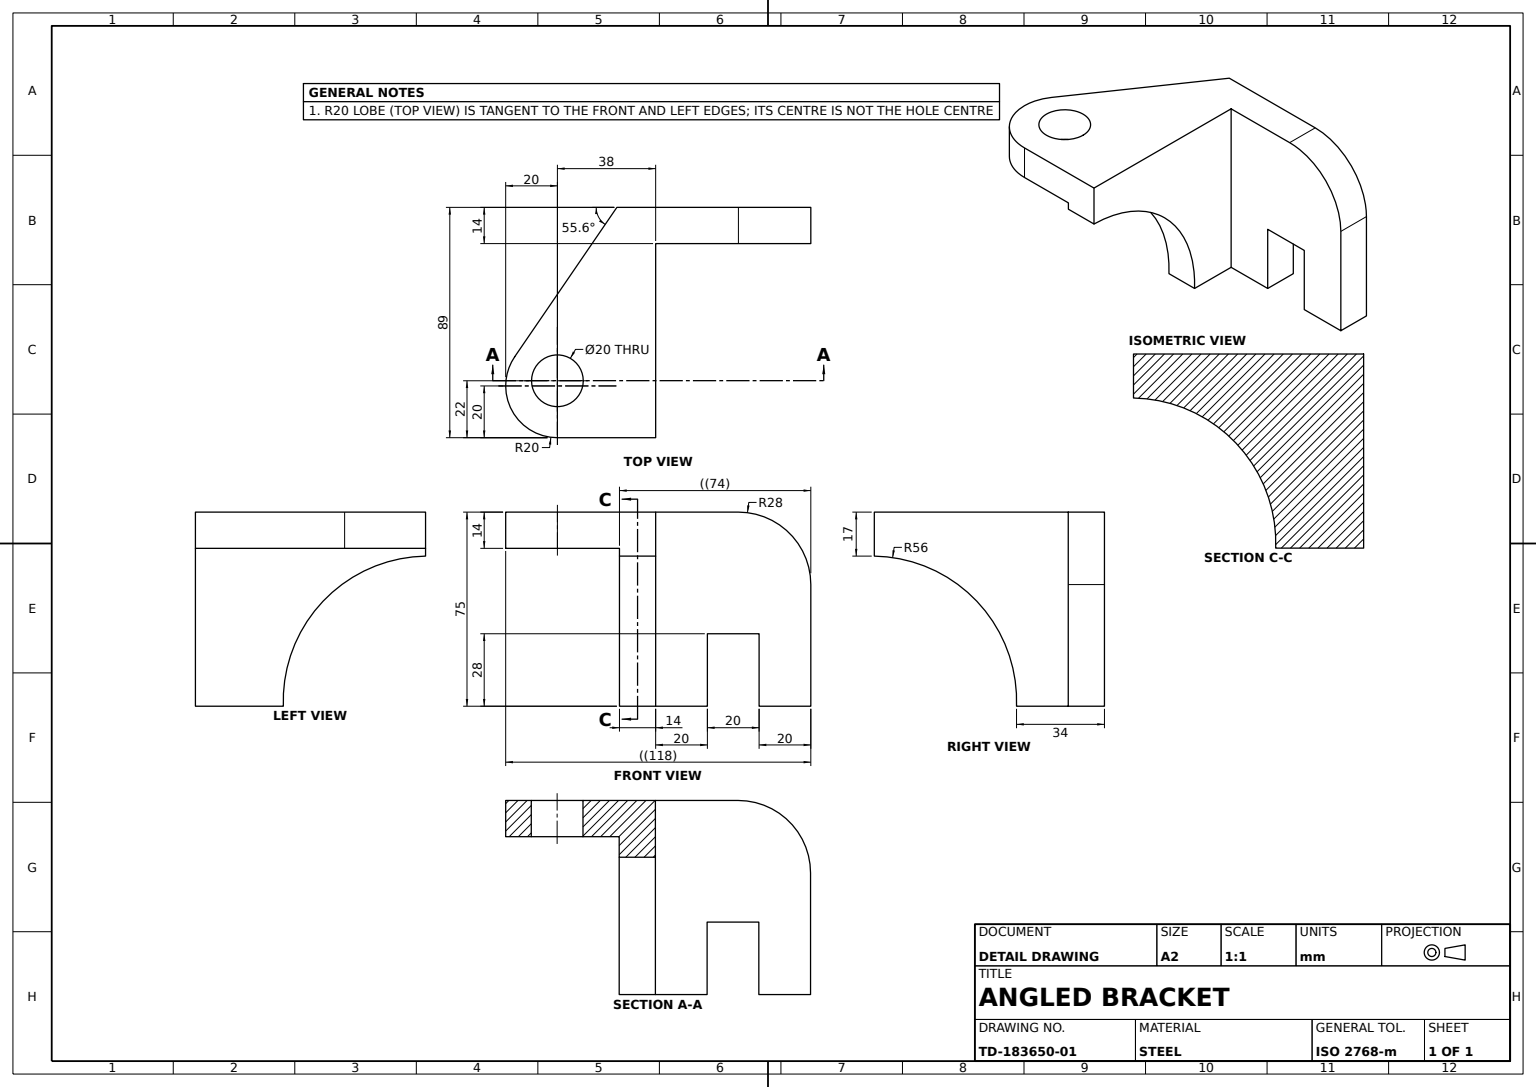
from build123d import *

# Parameters (mm, degrees)
BASE_PLATE_14MM_DEPTH  = 14
UPRIGHT_START          = 1
UPRIGHT_WEB_14MM_DEPTH = 14
SIDE_LUG_SKETCH_R      = 10
SIDE_LUG_14MM_DEPTH    = 14
CORNER_ROUND_R28_R     = 28


with BuildPart() as part:
    # Base Plate Sketch → Base Plate 14mm (new body)
    with BuildSketch(Plane.XY):
        Polygon((1, 0), (1, 75), (75, 75), (75, 0), (55, 0), (55, 28), (35, 28), (35, 0), align=None)
    extrude(amount=BASE_PLATE_14MM_DEPTH)

    # Upright Web Sketch → Upright Web 14mm (add)
    with BuildSketch(Plane(origin=(0, 0, 0), x_dir=(0, 0, -1), z_dir=(1, 0, 0)).offset(UPRIGHT_START)):
        with BuildLine():
            Line((-14, 75), (-89, 75))
            Line((-89, 75), (-89, 58))
            ThreePointArc((-89, 58), (-49.329041508, 40.541426156), (-34, 0))
            Line((-34, 0), (-14, 0))
            Line((-14, 0), (-14, 75))
        make_face()
    extrude(amount=UPRIGHT_WEB_14MM_DEPTH)

    # Side Lug Sketch → Side Lug 14mm (add)
    with BuildSketch(Plane(origin=(0, 75, 0), x_dir=(1, 0, 0), z_dir=(0, 1, 0))):
        with BuildLine():
            Line((1, -89), (-23, -89))
            ThreePointArc((-23, -89), (-40.691278494, -78.328379563), (-39.503096073, -57.701866526))
            Line((-39.503096073, -57.701866526), (0, 0))
            Line((0, 0), (1, 0))
            Line((1, 0), (1, -89))
        make_face()
        with Locations(Location((-23, -67, 0), (0, 0, 180))):
            Circle(SIDE_LUG_SKETCH_R, mode=Mode.SUBTRACT)
    extrude(amount=-SIDE_LUG_14MM_DEPTH)

    # Corner Round R28
    corner_round_r28_edges = [part.edges().sort_by_distance(p)[0] for p in [
        (75, 75, 7),
    ]]
    fillet(corner_round_r28_edges, radius=CORNER_ROUND_R28_R)


solid = part.part
